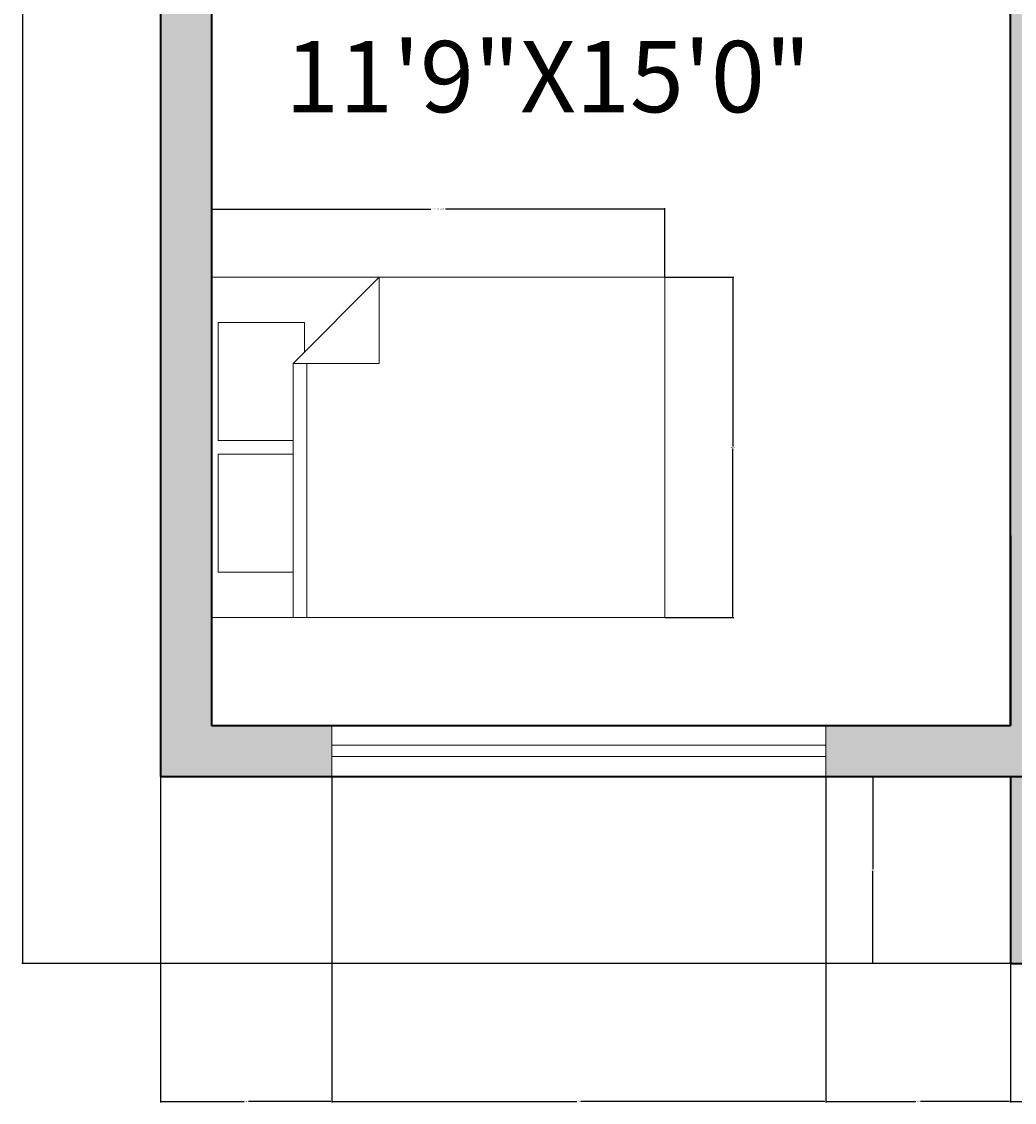
# Model space of a CAD drawing. Units: inches. Extents: x 582 to 1090, y 270 to 781.
# Tile 1 of 5: x 582 to 757, y 270 to 461. Entities that reach past the tile are written whole.
import ezdxf

# ---------------------------------------------------------------- set-up
doc = ezdxf.new("R2010")
doc.units = ezdxf.units.IN
doc.header["$MEASUREMENT"] = 0
for name, color, linetype, lineweight in [('A-ANNO-DIMS', 2, 'Continuous', 18), ('A-FURN', 8, 'Continuous', 18), ('A-GLAZ', 4, 'Continuous', 18), ('A-WALL', 7, 'Continuous', 35)]:
    doc.layers.add(name, color=color, linetype=linetype, lineweight=lineweight)
doc.layers.add('A-WALL-PATT', color=9, linetype='Continuous', lineweight=13, true_color=0xc7c8ca)
doc.styles.get("Standard").update_dxf_attribs({"font": 'arial.ttf'})
doc.dimstyles.get("Standard").update_dxf_attribs({"dimtxt": 0.18, "dimasz": 0.18, "dimexe": 0.18, "dimexo": 0.0625, "dimgap": 0.09, "dimtad": 0, "dimtih": 1, "dimtoh": 1, "dimdec": 0, "dimzin": 0, "dimdsep": 46, "dimlunit": 3, "dimtxsty": 'Standard', "dimcen": 0.09, "dimadec": 0, "dimazin": 0, "dimtfac": 1, "dimtdec": 0, "dimtofl": 0, "dimtmove": 0, "dimatfit": 3, "dimfxl": 1, "dimtolj": 1, "dimtzin": 0, "dimarcsym": 0})

# ---------------------------------------------------------------- blocks, each defined once
blk = doc.blocks.new('Bed - Queen')
for p, q in [((0, -80.00003), (0, 0)), ((0, 0), (59.99999, 0)), ((59.99999, 0), (59.99999, -80.00003)), ((7.99999, -1.2), (28.79998, -1.2)), ((7.99999, -14.4), (7.99999, -1.2)), ((28.79998, -1.2), (28.79998, -14.4)), ((31.19999, -1.2), (51.99999, -1.2)), ((31.19999, -14.4), (31.19999, -1.2)), ((51.99999, -1.2), (51.99999, -16.4)), ((0, -14.4), (44.8, -14.4)), ((59.99999, -29.6), (44.8, -14.4)), ((44.8, -14.4), (44.8, -29.6)), ((44.8, -16.8), (0, -16.8)), ((51.99999, -16.4), (46.79936, -16.4)), ((44.8, -29.6), (59.99999, -29.6)), ((59.99999, -80.00003), (0, -80.00003))]:
    blk.add_line(p, q)
blk = doc.blocks.new('*D10')
at = {"layer": 'A-ANNO-DIMS', "color": 0, "lineweight": -2, "transparency": 16777216}
for p, q in [((615.8, 415.56), (615.8, 427.67)), ((615.98, 427.49), (654.5, 427.49)), ((695.62, 427.49), (657.11, 427.49)), ((695.8, 415.56), (695.8, 427.67))]:
    blk.add_line(p, q, dxfattribs=at)
at = {"layer": 'A-ANNO-DIMS', "color": 0, "transparency": 16777216}
for points in [[(615.98, 427.52), (615.98, 427.46), (615.8, 427.49)], [(695.62, 427.52), (695.62, 427.46), (695.8, 427.49)]]:
    blk.add_solid(points, dxfattribs=at)
at = {"layer": 'Defpoints', "color": 0, "transparency": 16777216}
for p in [(615.8, 427.49), (615.8, 415.49), (695.8, 415.49)]:
    blk.add_point(p, dxfattribs=at)
at = {"layer": 'A-ANNO-DIMS', "color": 0, "transparency": 16777216, "insert": (655.8, 427.49), "char_height": 0.18, "attachment_point": 5}
blk.add_mtext('\\A1;QUEEN BED 80 TYP.', dxfattribs=at)
blk = doc.blocks.new('*D11')
at = {"layer": 'A-ANNO-DIMS', "color": 0, "lineweight": -2, "transparency": 16777216}
for p, q in [((695.87, 415.49), (707.98, 415.49)), ((707.8, 415.31), (707.8, 385.67)), ((707.8, 355.67), (707.8, 385.31)), ((695.87, 355.49), (707.98, 355.49))]:
    blk.add_line(p, q, dxfattribs=at)
at = {"layer": 'A-ANNO-DIMS', "color": 0, "transparency": 16777216}
for points in [[(707.77, 415.31), (707.83, 415.31), (707.8, 415.49)], [(707.77, 355.67), (707.83, 355.67), (707.8, 355.49)]]:
    blk.add_solid(points, dxfattribs=at)
at = {"layer": 'Defpoints', "color": 0, "transparency": 16777216}
for p in [(695.8, 415.49), (707.8, 415.49), (695.8, 355.49)]:
    blk.add_point(p, dxfattribs=at)
at = {"layer": 'A-ANNO-DIMS', "color": 0, "transparency": 16777216, "insert": (707.8, 385.49), "char_height": 0.18, "attachment_point": 5}
blk.add_mtext('\\A1;60 TYP.', dxfattribs=at)
blk = doc.blocks.new('*D36')
at = {"layer": 'A-ANNO-DIMS', "color": 0, "lineweight": -2, "transparency": 16777216}
for p, q in [((606.74, 744.45), (582.32, 744.45)), ((582.5, 744.27), (582.5, 519.62)), ((582.5, 294.62), (582.5, 519.26)), ((756.74, 294.44), (582.32, 294.44))]:
    blk.add_line(p, q, dxfattribs=at)
at = {"layer": 'A-ANNO-DIMS', "color": 0, "transparency": 16777216}
for points in [[(582.47, 744.27), (582.53, 744.27), (582.5, 744.45)], [(582.47, 294.62), (582.53, 294.62), (582.5, 294.44)]]:
    blk.add_solid(points, dxfattribs=at)
at = {"layer": 'Defpoints', "color": 0, "transparency": 16777216}
for p in [(582.5, 744.45), (606.8, 744.45), (756.8, 294.44)]:
    blk.add_point(p, dxfattribs=at)
at = {"layer": 'A-ANNO-DIMS', "color": 0, "transparency": 16777216, "insert": (582.5, 519.44), "char_height": 0.18, "attachment_point": 5}
blk.add_mtext('\\A1;450', dxfattribs=at)
blk = doc.blocks.new('*D37')
at = {"layer": 'A-ANNO-DIMS', "color": 0, "lineweight": -2, "transparency": 16777216}
for p, q in [((756.74, 327.45), (732.32, 327.45)), ((732.5, 327.27), (732.5, 311.12)), ((732.5, 294.62), (732.5, 310.76)), ((756.74, 294.44), (732.32, 294.44))]:
    blk.add_line(p, q, dxfattribs=at)
at = {"layer": 'A-ANNO-DIMS', "color": 0, "transparency": 16777216}
for points in [[(732.47, 327.27), (732.53, 327.27), (732.5, 327.45)], [(732.47, 294.62), (732.53, 294.62), (732.5, 294.44)]]:
    blk.add_solid(points, dxfattribs=at)
at = {"layer": 'Defpoints', "color": 0, "transparency": 16777216}
for p in [(732.5, 327.45), (756.8, 327.45), (756.8, 294.44)]:
    blk.add_point(p, dxfattribs=at)
at = {"layer": 'A-ANNO-DIMS', "color": 0, "transparency": 16777216, "insert": (732.5, 310.94), "char_height": 0.18, "attachment_point": 5}
blk.add_mtext('\\A1;33.01', dxfattribs=at)
blk = doc.blocks.new('*D39')
at = {"layer": 'A-ANNO-DIMS', "color": 0, "lineweight": -2, "transparency": 16777216}
for p, q in [((756.8, 294.37), (756.8, 269.96)), ((918.8, 294.37), (918.8, 269.96)), ((756.98, 270.14), (837.53, 270.14)), ((918.62, 270.14), (838.08, 270.14))]:
    blk.add_line(p, q, dxfattribs=at)
at = {"layer": 'A-ANNO-DIMS', "color": 0, "transparency": 16777216}
for points in [[(756.98, 270.17), (756.98, 270.11), (756.8, 270.14)], [(918.62, 270.17), (918.62, 270.11), (918.8, 270.14)]]:
    blk.add_solid(points, dxfattribs=at)
at = {"layer": 'Defpoints', "color": 0, "transparency": 16777216}
for p in [(756.8, 294.44), (918.8, 294.44), (918.8, 270.14)]:
    blk.add_point(p, dxfattribs=at)
at = {"layer": 'A-ANNO-DIMS', "color": 0, "transparency": 16777216, "insert": (837.8, 270.14), "char_height": 0.18, "attachment_point": 5}
blk.add_mtext('\\A1;162', dxfattribs=at)
blk = doc.blocks.new('*D40')
at = {"layer": 'A-ANNO-DIMS', "color": 0, "lineweight": -2, "transparency": 16777216}
for p, q in [((606.8, 327.38), (606.8, 269.96)), ((637.06, 327.38), (637.06, 269.96)), ((606.98, 270.14), (621.54, 270.14)), ((636.88, 270.14), (622.33, 270.14))]:
    blk.add_line(p, q, dxfattribs=at)
at = {"layer": 'A-ANNO-DIMS', "color": 0, "transparency": 16777216}
for points in [[(606.98, 270.17), (606.98, 270.11), (606.8, 270.14)], [(636.88, 270.17), (636.88, 270.11), (637.06, 270.14)]]:
    blk.add_solid(points, dxfattribs=at)
at = {"layer": 'Defpoints', "color": 0, "transparency": 16777216}
for p in [(606.8, 327.45), (637.06, 327.45), (637.06, 270.14)]:
    blk.add_point(p, dxfattribs=at)
at = {"layer": 'A-ANNO-DIMS', "color": 0, "transparency": 16777216, "insert": (621.93, 270.14), "char_height": 0.18, "attachment_point": 5}
blk.add_mtext('\\A1;30.26', dxfattribs=at)
blk = doc.blocks.new('*D41')
at = {"layer": 'A-ANNO-DIMS', "color": 0, "lineweight": -2, "transparency": 16777216}
for p, q in [((637.06, 327.38), (637.06, 269.96)), ((724.17, 327.38), (724.17, 269.96)), ((637.24, 270.14), (680.24, 270.14)), ((723.99, 270.14), (680.99, 270.14))]:
    blk.add_line(p, q, dxfattribs=at)
at = {"layer": 'A-ANNO-DIMS', "color": 0, "transparency": 16777216}
for points in [[(637.24, 270.17), (637.24, 270.11), (637.06, 270.14)], [(723.99, 270.17), (723.99, 270.11), (724.17, 270.14)]]:
    blk.add_solid(points, dxfattribs=at)
at = {"layer": 'Defpoints', "color": 0, "transparency": 16777216}
for p in [(637.06, 327.45), (724.17, 327.45), (724.17, 270.14)]:
    blk.add_point(p, dxfattribs=at)
at = {"layer": 'A-ANNO-DIMS', "color": 0, "transparency": 16777216, "insert": (680.62, 270.14), "char_height": 0.18, "attachment_point": 5}
blk.add_mtext('\\A1;87.11', dxfattribs=at)
blk = doc.blocks.new('*D42')
at = {"layer": 'A-ANNO-DIMS', "color": 0, "lineweight": -2, "transparency": 16777216}
for p, q in [((724.17, 327.38), (724.17, 269.96)), ((756.8, 327.38), (756.8, 269.96)), ((724.35, 270.14), (740.1, 270.14)), ((756.62, 270.14), (740.88, 270.14))]:
    blk.add_line(p, q, dxfattribs=at)
at = {"layer": 'A-ANNO-DIMS', "color": 0, "transparency": 16777216}
for points in [[(724.35, 270.17), (724.35, 270.11), (724.17, 270.14)], [(756.62, 270.17), (756.62, 270.11), (756.8, 270.14)]]:
    blk.add_solid(points, dxfattribs=at)
at = {"layer": 'Defpoints', "color": 0, "transparency": 16777216}
for p in [(724.17, 327.45), (756.8, 327.45), (756.8, 270.14)]:
    blk.add_point(p, dxfattribs=at)
at = {"layer": 'A-ANNO-DIMS', "color": 0, "transparency": 16777216, "insert": (740.49, 270.14), "char_height": 0.18, "attachment_point": 5}
blk.add_mtext('\\A1;32.63', dxfattribs=at)

msp = doc.modelspace()

# ---------------------------------------------------------------- hatches: boundary and pattern name
at = {"layer": 'A-WALL-PATT'}
h = msp.add_hatch(color=256, dxfattribs=at)
h.dxf.hatch_style = 1
h.paths.add_polyline_path([(867.8047, 744.446), (765.8047, 744.446), (606.8047, 744.446), (606.8047, 711.9379), (615.8047, 711.9379), (615.8047, 735.446), (756.8047, 735.446), (756.8047, 585.446), (765.8047, 585.446), (765.8047, 735.446), (868.9478, 735.446, -0.06325422)])
h.paths.add_polyline_path([(1065.8047, 744.446), (912.8047, 744.446), (903.8047, 744.446), (903.8047, 708.446), (903.8047, 594.446), (903.8047, 564.6071), (912.8047, 564.6071), (912.8047, 600.6071), (912.8047, 735.446), (1056.8047, 735.446), (1056.8047, 720.2375), (1065.8047, 720.2375)])
h.paths.add_polyline_path([(1065.8047, 632.4383), (1056.8047, 632.4383), (1056.8047, 594.446), (1056.8047, 584.9343), (1065.8047, 584.9343), (1065.8047, 594.446)], flags=17)
h.paths.add_polyline_path([(1056.8047, 603.446), (951.8047, 603.446), (951.8047, 594.446), (1056.8047, 594.446)], flags=17)
h.paths.add_polyline_path([(1065.8047, 525.446), (1065.8047, 550.2593), (1056.8047, 550.2593), (1056.8047, 534.446), (960.8047, 534.446), (960.8047, 565.946, -0.07397332), (952.1262, 564.6071), (951.8047, 564.6071), (951.8047, 495.446, -0.07632083), (960.8047, 494.0641), (960.8047, 525.446), (1056.8047, 525.446), (1056.8047, 508.8565), (1065.8047, 508.8565)])
h.paths.add_polyline_path([(1065.8047, 478.2143), (1056.8047, 478.2143), (1056.8047, 465.446), (951.8047, 465.446), (951.8047, 456.446), (1056.8047, 456.446), (1056.8047, 420.446), (1065.8047, 420.446), (1065.8047, 456.446)])
h.paths.add_polyline_path([(1065.8047, 420.446), (1056.8047, 420.446), (1017.8047, 420.446), (1017.8047, 456.446), (1008.8047, 456.446), (1008.8047, 411.446), (1038.8047, 411.446), (1065.8047, 411.446)])
h.paths.add_polyline_path([(1065.8047, 411.446), (1056.8047, 411.446), (1056.8047, 327.446), (1065.8047, 327.446)])
h.paths.add_polyline_path([(1065.8047, 327.446), (1056.8047, 327.446), (1017.8047, 327.446), (1017.8047, 382.8278, -0.07632083), (1008.8047, 381.446), (1008.8047, 327.446), (983.7348, 327.446), (983.7348, 318.446), (1065.8047, 318.446)])
h.paths.add_polyline_path([(946.9624, 327.446), (918.8047, 327.446), (918.8047, 369.8742), (918.8047, 459.446), (909.8047, 459.446), (909.8047, 369.8742), (909.8047, 318.446), (946.9624, 318.446)])
h.paths.add_polyline_path([(918.8047, 318.446), (909.8047, 318.446), (909.8047, 303.4372), (765.8047, 303.4372), (765.8047, 327.446), (756.8047, 327.446), (756.8047, 294.4372), (918.8047, 294.4372)])
h.paths.add_polyline_path([(909.8047, 378.8742), (882.3477, 378.8742), (882.3477, 347.0959), (889.3299, 347.0959), (889.3299, 369.8742), (909.8047, 369.8742)])
h.paths.add_polyline_path([(779.4225, 378.8742), (765.8047, 378.8742), (765.8047, 369.8742), (779.4225, 369.8742)])
h.paths.add_polyline_path([(765.8047, 516.446), (756.8047, 516.446), (756.8047, 480.446), (756.8047, 336.446), (724.1731, 336.446), (724.1731, 327.446), (765.8047, 327.446), (765.8047, 369.8742), (765.8047, 378.8742)])
h.paths.add_polyline_path([(615.8047, 516.446), (606.8047, 516.446), (606.8047, 327.446), (637.062, 327.446), (637.062, 336.446), (615.8047, 336.446)])
h.paths.add_polyline_path([(615.8047, 631.6498), (606.8047, 631.6498), (606.8047, 585.446), (606.8047, 569.338), (615.8047, 569.338), (615.8047, 585.446), (615.8047, 594.446)])
h.paths.add_polyline_path([(721.9478, 594.446), (615.8047, 594.446), (615.8047, 585.446), (627.9505, 585.446, -0.03261849), (629.8936, 585.446), (710.8047, 585.446), (710.8047, 525.446), (675.3033, 525.446), (675.3033, 516.446), (719.8047, 516.446), (720.8047, 516.446), (720.8047, 525.446), (719.8047, 525.446), (719.8047, 585.446), (720.8047, 585.446, -0.06325422)])
h.paths.add_polyline_path([(646.6852, 525.446), (615.8047, 525.446), (615.8047, 516.446), (645.3033, 516.446, -0.07632083)])
h.paths.add_polyline_path([(615.8047, 525.446), (615.8047, 539.7667), (606.8047, 539.7667), (606.8047, 516.446), (615.8047, 516.446)])

# ---------------------------------------------------------------- linework, layer by layer
at = {"layer": 'A-GLAZ'}
for p, q in [((637.062, 336.446), (637.062, 327.446)), ((724.1731, 331.946), (724.1731, 336.446)), ((724.1731, 336.446), (724.1731, 327.446)), ((637.062, 332.946), (724.1731, 332.946)), ((637.062, 330.946), (724.1731, 330.946))]:
    msp.add_line(p, q, dxfattribs=at)
at = {"layer": 'A-WALL'}
for p, q in [((606.8047, 516.446), (606.8047, 327.446)), ((615.8047, 516.446), (615.8047, 336.446)), ((756.8047, 336.446), (756.8047, 516.446)), ((756.8047, 369.8742), (756.8047, 336.446)), ((615.8047, 336.446), (756.8047, 336.446)), ((606.8047, 327.446), (765.8047, 327.446)), ((756.8047, 327.446), (756.8047, 294.4372)), ((756.8047, 294.4372), (918.8047, 294.4372))]:
    msp.add_line(p, q, dxfattribs=at)

# ---------------------------------------------------------------- block references
at = {"layer": 'A-FURN', "rotation": 90}
msp.add_blockref('Bed - Queen', (615.8047, 355.4925), dxfattribs=at)

# ---------------------------------------------------------------- texts
at = {"layer": 'A-ANNO-DIMS'}
msp.add_text('11\'9"X15\'0"', height=12.580749, dxfattribs=at).set_placement((628.7733, 444.6027))

# ---------------------------------------------------------------- dimensions: what is measured, and where the dimension line sits
for base, p2, override, picture, middle in [((582.5047, 744.446), (606.8047, 744.446), {"dimdec": 0, "dimlfac": 1, "dimrnd": 0, "dimzin": 0, "dimdsep": 46, "dimlunit": 2}, '*D36', (582.5047, 519.4416)), ((732.5047, 327.446), (756.8047, 327.446), {"dimdec": 2, "dimlfac": 1, "dimrnd": 0, "dimzin": 0, "dimdsep": 46, "dimlunit": 2}, '*D37', (732.5047, 310.9416))]:
    dim = msp.add_linear_dim(base=base, p1=(756.8047, 294.4372), p2=p2, angle=90, dimstyle='Standard', override=override, dxfattribs=at)
    dim.commit()
    dim.dimension.update_dxf_attribs({"geometry": picture, "text_midpoint": middle})
for base, p1, p2, angle, text, picture, middle in [((615.8047, 427.4925), (695.8047, 415.4925), (615.8047, 415.4925), 180, 'QUEEN BED <> TYP.', '*D10', (655.8047, 427.4925)), ((707.8047, 415.4925), (695.8047, 355.4925), (695.8047, 415.4925), 90, '<> TYP.', '*D11', (707.8047, 385.4925))]:
    dim = msp.add_linear_dim(base=base, p1=p1, p2=p2, angle=angle, text=text, dimstyle='Standard', override={"dimdec": 0, "dimlfac": 1, "dimrnd": 0, "dimzin": 0, "dimdsep": 46, "dimlunit": 2}, dxfattribs=at)
    dim.commit()
    dim.dimension.update_dxf_attribs({"geometry": picture, "text_midpoint": middle})
for base, p1, p2, override, picture, middle in [((637.062, 270.1372), (606.8047, 327.446), (637.062, 327.446), {"dimdec": 2, "dimlfac": 1, "dimrnd": 0, "dimzin": 0, "dimdsep": 46, "dimlunit": 2}, '*D40', (621.9334, 270.1372)), ((724.1731, 270.1372), (637.062, 327.446), (724.1731, 327.446), {"dimdec": 2, "dimlfac": 1, "dimrnd": 0, "dimzin": 0, "dimdsep": 46, "dimlunit": 2}, '*D41', (680.6175, 270.1372)), ((756.8047, 270.1372), (724.1731, 327.446), (756.8047, 327.446), {"dimdec": 2, "dimlfac": 1, "dimrnd": 0, "dimzin": 0, "dimdsep": 46, "dimlunit": 2}, '*D42', (740.4889, 270.1372)), ((918.8047, 270.1372), (756.8047, 294.4372), (918.8047, 294.4372), {"dimdec": 0, "dimlfac": 1, "dimrnd": 0, "dimzin": 0, "dimdsep": 46, "dimlunit": 2}, '*D39', (837.8047, 270.1372))]:
    dim = msp.add_linear_dim(base=base, p1=p1, p2=p2, dimstyle='Standard', override=override, dxfattribs=at)
    dim.commit()
    dim.dimension.update_dxf_attribs({"geometry": picture, "text_midpoint": middle})

doc.saveas('drawing.dxf')
